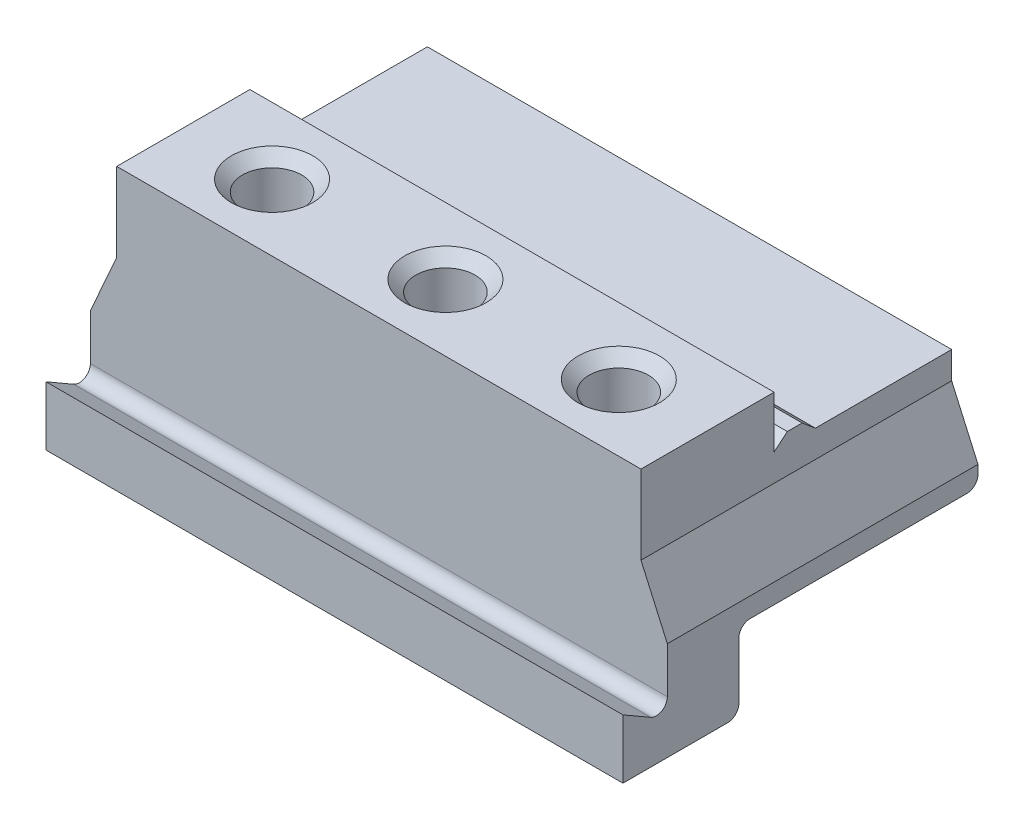
ISO-10303-21;
HEADER;
FILE_DESCRIPTION(('STEP AP214'),'2;1');
FILE_NAME('part.step','',(''),(''),'','','');
FILE_SCHEMA(('AUTOMOTIVE_DESIGN { 1 0 10303 214 1 1 1 1 }'));
ENDSEC;
DATA;
#1=APPLICATION_CONTEXT('core data for automotive mechanical design processes');
#2=APPLICATION_PROTOCOL_DEFINITION('international standard','automotive_design',2000,#1);
#3=PRODUCT_CONTEXT('',#1,'mechanical');
#4=PRODUCT('Part','Part','',(#3));
#5=PRODUCT_RELATED_PRODUCT_CATEGORY('part','',(#4));
#6=PRODUCT_DEFINITION_FORMATION('','',#4);
#7=PRODUCT_DEFINITION_CONTEXT('part definition',#1,'design');
#8=PRODUCT_DEFINITION('design','',#6,#7);
#9=PRODUCT_DEFINITION_SHAPE('','',#8);
#10=(LENGTH_UNIT() NAMED_UNIT(*) SI_UNIT(.MILLI.,.METRE.));
#11=(NAMED_UNIT(*) PLANE_ANGLE_UNIT() SI_UNIT($,.RADIAN.));
#12=(NAMED_UNIT(*) SI_UNIT($,.STERADIAN.) SOLID_ANGLE_UNIT());
#13=UNCERTAINTY_MEASURE_WITH_UNIT(LENGTH_MEASURE(1.E-05),#10,'distance_accuracy_value','');
#14=(GEOMETRIC_REPRESENTATION_CONTEXT(3) GLOBAL_UNCERTAINTY_ASSIGNED_CONTEXT((#13)) GLOBAL_UNIT_ASSIGNED_CONTEXT((#10,
#11,#12)) REPRESENTATION_CONTEXT('',''));
#15=CARTESIAN_POINT('',(0.,0.,0.));
#16=DIRECTION('',(0.,0.,1.));
#17=DIRECTION('',(1.,0.,0.));
#18=AXIS2_PLACEMENT_3D('',#15,#16,#17);
#19=CARTESIAN_POINT('',(78.,0.,-48.));
#20=DIRECTION('',(0.,-1.,0.));
#21=DIRECTION('',(1.,0.,0.));
#22=AXIS2_PLACEMENT_3D('',#19,#20,#21);
#23=PLANE('',#22);
#24=DIRECTION('',(0.,0.,1.));
#25=VECTOR('',#24,1.);
#26=CARTESIAN_POINT('',(0.,0.,-48.));
#27=LINE('',#26,#25);
#28=CARTESIAN_POINT('',(0.,0.,-14.1713819919104));
#29=VERTEX_POINT('',#28);
#30=CARTESIAN_POINT('',(0.,0.,0.));
#31=VERTEX_POINT('',#30);
#32=EDGE_CURVE('E197',#29,#31,#27,.T.);
#33=ORIENTED_EDGE('',*,*,#32,.F.);
#34=DIRECTION('',(1.,0.,0.));
#35=VECTOR('',#34,1.);
#36=CARTESIAN_POINT('',(-9.99999999999999,0.,-14.1713819919104));
#37=LINE('',#36,#35);
#38=CARTESIAN_POINT('',(78.,0.,-14.1713819919104));
#39=VERTEX_POINT('',#38);
#40=EDGE_CURVE('E409',#29,#39,#37,.T.);
#41=ORIENTED_EDGE('',*,*,#40,.T.);
#42=DIRECTION('',(0.,0.,1.));
#43=VECTOR('',#42,1.);
#44=CARTESIAN_POINT('',(78.,0.,-48.));
#45=LINE('',#44,#43);
#46=CARTESIAN_POINT('',(78.,0.,0.));
#47=VERTEX_POINT('',#46);
#48=EDGE_CURVE('E243',#39,#47,#45,.T.);
#49=ORIENTED_EDGE('',*,*,#48,.T.);
#50=DIRECTION('',(1.,0.,0.));
#51=VECTOR('',#50,1.);
#52=CARTESIAN_POINT('',(78.,0.,0.));
#53=LINE('',#52,#51);
#54=EDGE_CURVE('E213',#31,#47,#53,.T.);
#55=ORIENTED_EDGE('',*,*,#54,.F.);
#56=EDGE_LOOP('',(#33,#41,#49,#55));
#57=FACE_BOUND('',#56,.T.);
#58=ADVANCED_FACE('F41',(#57),#23,.T.);
#59=CARTESIAN_POINT('',(0.,0.,-48.));
#60=DIRECTION('',(-1.,0.,0.));
#61=DIRECTION('',(0.,0.,1.));
#62=AXIS2_PLACEMENT_3D('',#59,#60,#61);
#63=PLANE('',#62);
#64=DIRECTION('',(0.,-1.,0.));
#65=VECTOR('',#64,1.);
#66=CARTESIAN_POINT('',(0.,0.,-6.));
#67=LINE('',#66,#65);
#68=CARTESIAN_POINT('',(0.,13.33,-6.));
#69=VERTEX_POINT('',#68);
#70=CARTESIAN_POINT('',(0.,7.13397459621554,-6.));
#71=VERTEX_POINT('',#70);
#72=EDGE_CURVE('E490',#69,#71,#67,.T.);
#73=ORIENTED_EDGE('',*,*,#72,.F.);
#74=DIRECTION('',(0.,0.,1.));
#75=VECTOR('',#74,1.);
#76=CARTESIAN_POINT('',(0.,13.33,-48.));
#77=LINE('',#76,#75);
#78=CARTESIAN_POINT('',(0.,13.33,-48.));
#79=VERTEX_POINT('',#78);
#80=EDGE_CURVE('E224',#79,#69,#77,.T.);
#81=ORIENTED_EDGE('',*,*,#80,.F.);
#82=DIRECTION('',(0.,-1.,0.));
#83=VECTOR('',#82,1.);
#84=CARTESIAN_POINT('',(0.,0.,-48.));
#85=LINE('',#84,#83);
#86=CARTESIAN_POINT('',(0.,12.17,-48.));
#87=VERTEX_POINT('',#86);
#88=EDGE_CURVE('E242',#79,#87,#85,.T.);
#89=ORIENTED_EDGE('',*,*,#88,.T.);
#90=CARTESIAN_POINT('',(0.,12.17,-46.5));
#91=DIRECTION('',(-1.,0.,0.));
#92=DIRECTION('',(0.,0.,1.));
#93=AXIS2_PLACEMENT_3D('',#90,#91,#92);
#94=CIRCLE('',#93,1.5);
#95=CARTESIAN_POINT('',(0.,10.67,-46.5));
#96=VERTEX_POINT('',#95);
#97=EDGE_CURVE('E63',#96,#87,#94,.F.);
#98=ORIENTED_EDGE('',*,*,#97,.F.);
#99=DIRECTION('',(0.,0.,-1.));
#100=VECTOR('',#99,1.);
#101=CARTESIAN_POINT('',(0.,10.67,-48.));
#102=LINE('',#101,#100);
#103=CARTESIAN_POINT('',(0.,10.67,-17.1713819919104));
#104=VERTEX_POINT('',#103);
#105=EDGE_CURVE('E469',#104,#96,#102,.T.);
#106=ORIENTED_EDGE('',*,*,#105,.F.);
#107=CARTESIAN_POINT('',(0.,9.17,-17.1713819919104));
#108=DIRECTION('',(-1.,0.,0.));
#109=DIRECTION('',(0.,0.,1.));
#110=AXIS2_PLACEMENT_3D('',#107,#108,#109);
#111=CIRCLE('',#110,1.5);
#112=CARTESIAN_POINT('',(0.,9.16999999999999,-15.6713819919104));
#113=VERTEX_POINT('',#112);
#114=EDGE_CURVE('E472',#104,#113,#111,.F.);
#115=ORIENTED_EDGE('',*,*,#114,.T.);
#116=DIRECTION('',(0.,1.,0.));
#117=VECTOR('',#116,1.);
#118=CARTESIAN_POINT('',(0.,0.,-15.6713819919104));
#119=LINE('',#118,#117);
#120=CARTESIAN_POINT('',(0.,1.50000000000001,-15.6713819919104));
#121=VERTEX_POINT('',#120);
#122=EDGE_CURVE('E471',#121,#113,#119,.T.);
#123=ORIENTED_EDGE('',*,*,#122,.F.);
#124=CARTESIAN_POINT('',(0.,1.5,-14.1713819919104));
#125=DIRECTION('',(-1.,0.,0.));
#126=DIRECTION('',(0.,0.,1.));
#127=AXIS2_PLACEMENT_3D('',#124,#125,#126);
#128=CIRCLE('',#127,1.5);
#129=EDGE_CURVE('E479',#121,#29,#128,.T.);
#130=ORIENTED_EDGE('',*,*,#129,.T.);
#131=ORIENTED_EDGE('',*,*,#32,.T.);
#132=DIRECTION('',(0.,-1.,0.));
#133=VECTOR('',#132,1.);
#134=CARTESIAN_POINT('',(0.,0.,0.));
#135=LINE('',#134,#133);
#136=CARTESIAN_POINT('',(0.,8.,0.));
#137=VERTEX_POINT('',#136);
#138=EDGE_CURVE('E219',#137,#31,#135,.T.);
#139=ORIENTED_EDGE('',*,*,#138,.F.);
#140=DIRECTION('',(0.,0.500000000000004,0.866025403784436));
#141=VECTOR('',#140,1.);
#142=CARTESIAN_POINT('',(0.,-14.7846096908267,-39.4641016151376));
#143=LINE('',#142,#141);
#144=CARTESIAN_POINT('',(0.,5.83493649053889,-3.74999999999999));
#145=VERTEX_POINT('',#144);
#146=EDGE_CURVE('E191',#145,#137,#143,.T.);
#147=ORIENTED_EDGE('',*,*,#146,.F.);
#148=CARTESIAN_POINT('',(0.,7.13397459621554,-4.5));
#149=DIRECTION('',(-1.,0.,0.));
#150=DIRECTION('',(0.,0.,1.));
#151=AXIS2_PLACEMENT_3D('',#148,#149,#150);
#152=CIRCLE('',#151,1.5);
#153=EDGE_CURVE('E478',#71,#145,#152,.T.);
#154=ORIENTED_EDGE('',*,*,#153,.F.);
#155=EDGE_LOOP('',(#73,#81,#89,#98,#106,#115,#123,#130,#131,#139,#147,#154));
#156=FACE_BOUND('',#155,.T.);
#157=ADVANCED_FACE('F287',(#156),#63,.T.);
#158=CARTESIAN_POINT('',(78.,13.33,-48.));
#159=DIRECTION('',(1.,0.,0.));
#160=DIRECTION('',(0.,0.,-1.));
#161=AXIS2_PLACEMENT_3D('',#158,#159,#160);
#162=PLANE('',#161);
#163=DIRECTION('',(0.,1.,0.));
#164=VECTOR('',#163,1.);
#165=CARTESIAN_POINT('',(78.,7.13397459621554,-6.));
#166=LINE('',#165,#164);
#167=CARTESIAN_POINT('',(78.,7.13397459621554,-6.));
#168=VERTEX_POINT('',#167);
#169=CARTESIAN_POINT('',(78.,13.33,-6.));
#170=VERTEX_POINT('',#169);
#171=EDGE_CURVE('E423',#168,#170,#166,.T.);
#172=ORIENTED_EDGE('',*,*,#171,.F.);
#173=CARTESIAN_POINT('',(78.,7.13397459621554,-4.5));
#174=DIRECTION('',(1.,0.,0.));
#175=DIRECTION('',(0.,0.,-1.));
#176=AXIS2_PLACEMENT_3D('',#173,#174,#175);
#177=CIRCLE('',#176,1.5);
#178=CARTESIAN_POINT('',(78.,5.83493649053889,-3.74999999999999));
#179=VERTEX_POINT('',#178);
#180=EDGE_CURVE('E208',#179,#168,#177,.T.);
#181=ORIENTED_EDGE('',*,*,#180,.F.);
#182=DIRECTION('',(0.,-0.500000000000004,-0.866025403784436));
#183=VECTOR('',#182,1.);
#184=CARTESIAN_POINT('',(78.,8.,0.));
#185=LINE('',#184,#183);
#186=CARTESIAN_POINT('',(78.,8.,0.));
#187=VERTEX_POINT('',#186);
#188=EDGE_CURVE('E192',#187,#179,#185,.T.);
#189=ORIENTED_EDGE('',*,*,#188,.F.);
#190=DIRECTION('',(0.,1.,0.));
#191=VECTOR('',#190,1.);
#192=CARTESIAN_POINT('',(78.,13.33,0.));
#193=LINE('',#192,#191);
#194=EDGE_CURVE('E210',#47,#187,#193,.T.);
#195=ORIENTED_EDGE('',*,*,#194,.F.);
#196=ORIENTED_EDGE('',*,*,#48,.F.);
#197=CARTESIAN_POINT('',(78.,1.5,-14.1713819919104));
#198=DIRECTION('',(1.,0.,0.));
#199=DIRECTION('',(0.,0.,-1.));
#200=AXIS2_PLACEMENT_3D('',#197,#198,#199);
#201=CIRCLE('',#200,1.5);
#202=CARTESIAN_POINT('',(78.,1.50000000000001,-15.6713819919104));
#203=VERTEX_POINT('',#202);
#204=EDGE_CURVE('E444',#39,#203,#201,.T.);
#205=ORIENTED_EDGE('',*,*,#204,.T.);
#206=DIRECTION('',(0.,-1.,0.));
#207=VECTOR('',#206,1.);
#208=CARTESIAN_POINT('',(78.,9.16999999999999,-15.6713819919104));
#209=LINE('',#208,#207);
#210=CARTESIAN_POINT('',(78.,9.16999999999999,-15.6713819919104));
#211=VERTEX_POINT('',#210);
#212=EDGE_CURVE('E454',#211,#203,#209,.T.);
#213=ORIENTED_EDGE('',*,*,#212,.F.);
#214=CARTESIAN_POINT('',(78.,9.17,-17.1713819919104));
#215=DIRECTION('',(-1.,0.,0.));
#216=DIRECTION('',(0.,0.,1.));
#217=AXIS2_PLACEMENT_3D('',#214,#215,#216);
#218=CIRCLE('',#217,1.5);
#219=CARTESIAN_POINT('',(78.,10.67,-17.1713819919104));
#220=VERTEX_POINT('',#219);
#221=EDGE_CURVE('E459',#211,#220,#218,.T.);
#222=ORIENTED_EDGE('',*,*,#221,.T.);
#223=DIRECTION('',(0.,0.,1.));
#224=VECTOR('',#223,1.);
#225=CARTESIAN_POINT('',(78.,10.67,-46.5));
#226=LINE('',#225,#224);
#227=CARTESIAN_POINT('',(78.,10.67,-46.5));
#228=VERTEX_POINT('',#227);
#229=EDGE_CURVE('E458',#228,#220,#226,.T.);
#230=ORIENTED_EDGE('',*,*,#229,.F.);
#231=CARTESIAN_POINT('',(78.,12.17,-46.5));
#232=DIRECTION('',(-1.,0.,0.));
#233=DIRECTION('',(0.,0.,1.));
#234=AXIS2_PLACEMENT_3D('',#231,#232,#233);
#235=CIRCLE('',#234,1.5);
#236=CARTESIAN_POINT('',(78.,12.17,-48.));
#237=VERTEX_POINT('',#236);
#238=EDGE_CURVE('E445',#237,#228,#235,.T.);
#239=ORIENTED_EDGE('',*,*,#238,.F.);
#240=DIRECTION('',(0.,1.,0.));
#241=VECTOR('',#240,1.);
#242=CARTESIAN_POINT('',(78.,13.33,-48.));
#243=LINE('',#242,#241);
#244=CARTESIAN_POINT('',(78.,13.33,-48.));
#245=VERTEX_POINT('',#244);
#246=EDGE_CURVE('E220',#237,#245,#243,.T.);
#247=ORIENTED_EDGE('',*,*,#246,.T.);
#248=DIRECTION('',(0.,0.,1.));
#249=VECTOR('',#248,1.);
#250=CARTESIAN_POINT('',(78.,13.33,-48.));
#251=LINE('',#250,#249);
#252=EDGE_CURVE('E239',#245,#170,#251,.T.);
#253=ORIENTED_EDGE('',*,*,#252,.T.);
#254=EDGE_LOOP('',(#172,#181,#189,#195,#196,#205,#213,#222,#230,#239,#247,#253));
#255=FACE_BOUND('',#254,.T.);
#256=ADVANCED_FACE('F204',(#255),#162,.T.);
#257=CARTESIAN_POINT('',(0.,0.,-48.));
#258=DIRECTION('',(0.,0.,-1.));
#259=DIRECTION('',(-1.,0.,0.));
#260=AXIS2_PLACEMENT_3D('',#257,#258,#259);
#261=PLANE('',#260);
#262=DIRECTION('',(-1.,0.,0.));
#263=VECTOR('',#262,1.);
#264=CARTESIAN_POINT('',(0.,25.,-48.));
#265=LINE('',#264,#263);
#266=CARTESIAN_POINT('',(74.4381705175317,25.,-48.));
#267=VERTEX_POINT('',#266);
#268=CARTESIAN_POINT('',(3.5618294824683,25.,-48.));
#269=VERTEX_POINT('',#268);
#270=EDGE_CURVE('E250',#267,#269,#265,.T.);
#271=ORIENTED_EDGE('',*,*,#270,.F.);
#272=DIRECTION('',(0.,1.,0.));
#273=VECTOR('',#272,1.);
#274=CARTESIAN_POINT('',(74.4381705175317,32.,-48.));
#275=LINE('',#274,#273);
#276=CARTESIAN_POINT('',(74.4381705175317,21.33,-48.));
#277=VERTEX_POINT('',#276);
#278=EDGE_CURVE('E505',#277,#267,#275,.T.);
#279=ORIENTED_EDGE('',*,*,#278,.F.);
#280=DIRECTION('',(-0.4067366430758,0.913545457642601,0.));
#281=VECTOR('',#280,1.);
#282=CARTESIAN_POINT('',(74.4381705175317,21.33,-48.));
#283=LINE('',#282,#281);
#284=EDGE_CURVE('E497',#245,#277,#283,.T.);
#285=ORIENTED_EDGE('',*,*,#284,.F.);
#286=ORIENTED_EDGE('',*,*,#246,.F.);
#287=DIRECTION('',(1.,0.,0.));
#288=VECTOR('',#287,1.);
#289=CARTESIAN_POINT('',(-9.99999999999999,12.17,-48.));
#290=LINE('',#289,#288);
#291=EDGE_CURVE('E198',#237,#87,#290,.F.);
#292=ORIENTED_EDGE('',*,*,#291,.T.);
#293=ORIENTED_EDGE('',*,*,#88,.F.);
#294=DIRECTION('',(-0.406736643075801,-0.913545457642601,0.));
#295=VECTOR('',#294,1.);
#296=CARTESIAN_POINT('',(0.,13.33,-48.));
#297=LINE('',#296,#295);
#298=CARTESIAN_POINT('',(3.5618294824683,21.33,-48.));
#299=VERTEX_POINT('',#298);
#300=EDGE_CURVE('E510',#299,#79,#297,.T.);
#301=ORIENTED_EDGE('',*,*,#300,.F.);
#302=DIRECTION('',(0.,-1.,0.));
#303=VECTOR('',#302,1.);
#304=CARTESIAN_POINT('',(3.5618294824683,21.33,-48.));
#305=LINE('',#304,#303);
#306=EDGE_CURVE('E504',#269,#299,#305,.T.);
#307=ORIENTED_EDGE('',*,*,#306,.F.);
#308=EDGE_LOOP('',(#271,#279,#285,#286,#292,#293,#301,#307));
#309=FACE_BOUND('',#308,.T.);
#310=ADVANCED_FACE('F308',(#309),#261,.T.);
#311=CARTESIAN_POINT('',(0.,13.33,-48.));
#312=DIRECTION('',(-0.9135454576426,0.406736643075801,0.));
#313=DIRECTION('',(-0.406736643075801,-0.913545457642601,0.));
#314=AXIS2_PLACEMENT_3D('',#311,#312,#313);
#315=PLANE('',#314);
#316=DIRECTION('',(-0.406736643075801,-0.913545457642601,0.));
#317=VECTOR('',#316,1.);
#318=CARTESIAN_POINT('',(0.,13.33,-6.));
#319=LINE('',#318,#317);
#320=CARTESIAN_POINT('',(3.5618294824683,21.33,-6.));
#321=VERTEX_POINT('',#320);
#322=EDGE_CURVE('E487',#321,#69,#319,.T.);
#323=ORIENTED_EDGE('',*,*,#322,.F.);
#324=DIRECTION('',(0.,0.,1.));
#325=VECTOR('',#324,1.);
#326=CARTESIAN_POINT('',(3.5618294824683,21.33,-48.));
#327=LINE('',#326,#325);
#328=EDGE_CURVE('E226',#299,#321,#327,.T.);
#329=ORIENTED_EDGE('',*,*,#328,.F.);
#330=ORIENTED_EDGE('',*,*,#300,.T.);
#331=ORIENTED_EDGE('',*,*,#80,.T.);
#332=EDGE_LOOP('',(#323,#329,#330,#331));
#333=FACE_BOUND('',#332,.T.);
#334=ADVANCED_FACE('F321',(#333),#315,.T.);
#335=CARTESIAN_POINT('',(3.5618294824683,21.33,-48.));
#336=DIRECTION('',(-1.,0.,0.));
#337=DIRECTION('',(0.,0.,1.));
#338=AXIS2_PLACEMENT_3D('',#335,#336,#337);
#339=PLANE('',#338);
#340=DIRECTION('',(0.,-1.,0.));
#341=VECTOR('',#340,1.);
#342=CARTESIAN_POINT('',(3.5618294824683,21.33,-6.));
#343=LINE('',#342,#341);
#344=CARTESIAN_POINT('',(3.5618294824683,32.,-6.));
#345=VERTEX_POINT('',#344);
#346=EDGE_CURVE('E484',#345,#321,#343,.T.);
#347=ORIENTED_EDGE('',*,*,#346,.F.);
#348=DIRECTION('',(0.,0.,1.));
#349=VECTOR('',#348,1.);
#350=CARTESIAN_POINT('',(3.5618294824683,32.,-48.));
#351=LINE('',#350,#349);
#352=CARTESIAN_POINT('',(3.5618294824683,32.,-24.));
#353=VERTEX_POINT('',#352);
#354=EDGE_CURVE('E233',#353,#345,#351,.T.);
#355=ORIENTED_EDGE('',*,*,#354,.F.);
#356=DIRECTION('',(0.,1.,0.));
#357=VECTOR('',#356,1.);
#358=CARTESIAN_POINT('',(3.5618294824683,21.33,-24.));
#359=LINE('',#358,#357);
#360=CARTESIAN_POINT('',(3.5618294824683,25.,-24.));
#361=VERTEX_POINT('',#360);
#362=EDGE_CURVE('E493',#361,#353,#359,.T.);
#363=ORIENTED_EDGE('',*,*,#362,.F.);
#364=DIRECTION('',(0.,-0.642787609686541,0.766044443118977));
#365=VECTOR('',#364,1.);
#366=CARTESIAN_POINT('',(3.5618294824683,35.3013374421653,-36.2766559052257));
#367=LINE('',#366,#365);
#368=CARTESIAN_POINT('',(3.5618294824683,26.5,-25.7876303888913));
#369=VERTEX_POINT('',#368);
#370=EDGE_CURVE('E491',#369,#361,#367,.T.);
#371=ORIENTED_EDGE('',*,*,#370,.F.);
#372=DIRECTION('',(0.,0.,1.));
#373=VECTOR('',#372,1.);
#374=CARTESIAN_POINT('',(3.5618294824683,26.5,-48.));
#375=LINE('',#374,#373);
#376=CARTESIAN_POINT('',(3.5618294824683,26.5,-27.7876303888913));
#377=VERTEX_POINT('',#376);
#378=EDGE_CURVE('E492',#377,#369,#375,.T.);
#379=ORIENTED_EDGE('',*,*,#378,.F.);
#380=DIRECTION('',(0.,0.642787609686539,0.766044443118978));
#381=VECTOR('',#380,1.);
#382=CARTESIAN_POINT('',(3.5618294824683,14.4112313893849,-42.1944638106319));
#383=LINE('',#382,#381);
#384=CARTESIAN_POINT('',(3.5618294824683,25.,-29.5752607777826));
#385=VERTEX_POINT('',#384);
#386=EDGE_CURVE('E217',#385,#377,#383,.T.);
#387=ORIENTED_EDGE('',*,*,#386,.F.);
#388=DIRECTION('',(0.,0.,1.));
#389=VECTOR('',#388,1.);
#390=CARTESIAN_POINT('',(3.5618294824683,25.,-48.));
#391=LINE('',#390,#389);
#392=EDGE_CURVE('E470',#269,#385,#391,.T.);
#393=ORIENTED_EDGE('',*,*,#392,.F.);
#394=ORIENTED_EDGE('',*,*,#306,.T.);
#395=ORIENTED_EDGE('',*,*,#328,.T.);
#396=EDGE_LOOP('',(#347,#355,#363,#371,#379,#387,#393,#394,#395));
#397=FACE_BOUND('',#396,.T.);
#398=ADVANCED_FACE('F318',(#397),#339,.T.);
#399=CARTESIAN_POINT('',(3.5618294824683,32.,-48.));
#400=DIRECTION('',(0.,1.,0.));
#401=DIRECTION('',(0.,0.,1.));
#402=AXIS2_PLACEMENT_3D('',#399,#400,#401);
#403=PLANE('',#402);
#404=CARTESIAN_POINT('',(62.4381705175317,32.,-15.));
#405=DIRECTION('',(0.,1.,0.));
#406=DIRECTION('',(0.,0.,1.));
#407=AXIS2_PLACEMENT_3D('',#404,#405,#406);
#408=CIRCLE('',#407,5.5);
#409=CARTESIAN_POINT('',(62.4381705175317,32.,-9.49999999999999));
#410=VERTEX_POINT('',#409);
#411=EDGE_CURVE('E266',#410,#410,#408,.F.);
#412=ORIENTED_EDGE('',*,*,#411,.T.);
#413=EDGE_LOOP('',(#412));
#414=FACE_BOUND('',#413,.T.);
#415=CARTESIAN_POINT('',(39.,32.,-15.));
#416=DIRECTION('',(0.,1.,0.));
#417=DIRECTION('',(0.,0.,1.));
#418=AXIS2_PLACEMENT_3D('',#415,#416,#417);
#419=CIRCLE('',#418,5.49999999999998);
#420=CARTESIAN_POINT('',(39.,32.,-9.50000000000002));
#421=VERTEX_POINT('',#420);
#422=EDGE_CURVE('E265',#421,#421,#419,.F.);
#423=ORIENTED_EDGE('',*,*,#422,.T.);
#424=EDGE_LOOP('',(#423));
#425=FACE_BOUND('',#424,.T.);
#426=CARTESIAN_POINT('',(15.5618294824683,32.,-15.));
#427=DIRECTION('',(0.,1.,0.));
#428=DIRECTION('',(0.,0.,1.));
#429=AXIS2_PLACEMENT_3D('',#426,#427,#428);
#430=CIRCLE('',#429,5.49999999999998);
#431=CARTESIAN_POINT('',(15.5618294824683,32.,-9.50000000000002));
#432=VERTEX_POINT('',#431);
#433=EDGE_CURVE('E258',#432,#432,#430,.F.);
#434=ORIENTED_EDGE('',*,*,#433,.T.);
#435=EDGE_LOOP('',(#434));
#436=FACE_BOUND('',#435,.T.);
#437=DIRECTION('',(1.,0.,0.));
#438=VECTOR('',#437,1.);
#439=CARTESIAN_POINT('',(-9.99999999999999,32.,-6.));
#440=LINE('',#439,#438);
#441=CARTESIAN_POINT('',(74.4381705175317,32.,-6.));
#442=VERTEX_POINT('',#441);
#443=EDGE_CURVE('E425',#345,#442,#440,.T.);
#444=ORIENTED_EDGE('',*,*,#443,.T.);
#445=DIRECTION('',(0.,0.,1.));
#446=VECTOR('',#445,1.);
#447=CARTESIAN_POINT('',(74.4381705175317,32.,-48.));
#448=LINE('',#447,#446);
#449=CARTESIAN_POINT('',(74.4381705175317,32.,-24.));
#450=VERTEX_POINT('',#449);
#451=EDGE_CURVE('E234',#450,#442,#448,.T.);
#452=ORIENTED_EDGE('',*,*,#451,.F.);
#453=DIRECTION('',(1.,0.,0.));
#454=VECTOR('',#453,1.);
#455=CARTESIAN_POINT('',(-9.99999999999999,32.,-24.));
#456=LINE('',#455,#454);
#457=EDGE_CURVE('E212',#353,#450,#456,.T.);
#458=ORIENTED_EDGE('',*,*,#457,.F.);
#459=ORIENTED_EDGE('',*,*,#354,.T.);
#460=EDGE_LOOP('',(#444,#452,#458,#459));
#461=FACE_BOUND('',#460,.T.);
#462=ADVANCED_FACE('F317',(#414,#425,#436,#461),#403,.T.);
#463=CARTESIAN_POINT('',(74.4381705175317,32.,-48.));
#464=DIRECTION('',(1.,0.,0.));
#465=DIRECTION('',(0.,0.,-1.));
#466=AXIS2_PLACEMENT_3D('',#463,#464,#465);
#467=PLANE('',#466);
#468=DIRECTION('',(0.,1.,0.));
#469=VECTOR('',#468,1.);
#470=CARTESIAN_POINT('',(74.4381705175317,32.,-6.));
#471=LINE('',#470,#469);
#472=CARTESIAN_POINT('',(74.4381705175317,21.33,-6.));
#473=VERTEX_POINT('',#472);
#474=EDGE_CURVE('E483',#473,#442,#471,.T.);
#475=ORIENTED_EDGE('',*,*,#474,.F.);
#476=DIRECTION('',(0.,0.,1.));
#477=VECTOR('',#476,1.);
#478=CARTESIAN_POINT('',(74.4381705175317,21.33,-48.));
#479=LINE('',#478,#477);
#480=EDGE_CURVE('E240',#277,#473,#479,.T.);
#481=ORIENTED_EDGE('',*,*,#480,.F.);
#482=ORIENTED_EDGE('',*,*,#278,.T.);
#483=DIRECTION('',(0.,0.,-1.));
#484=VECTOR('',#483,1.);
#485=CARTESIAN_POINT('',(74.4381705175317,25.,-48.));
#486=LINE('',#485,#484);
#487=CARTESIAN_POINT('',(74.4381705175317,25.,-29.5752607777826));
#488=VERTEX_POINT('',#487);
#489=EDGE_CURVE('E60',#488,#267,#486,.T.);
#490=ORIENTED_EDGE('',*,*,#489,.F.);
#491=DIRECTION('',(0.,-0.642787609686539,-0.766044443118978));
#492=VECTOR('',#491,1.);
#493=CARTESIAN_POINT('',(74.4381705175317,18.8198183615318,-36.9405144483118));
#494=LINE('',#493,#492);
#495=CARTESIAN_POINT('',(74.4381705175317,26.5,-27.7876303888913));
#496=VERTEX_POINT('',#495);
#497=EDGE_CURVE('E253',#496,#488,#494,.T.);
#498=ORIENTED_EDGE('',*,*,#497,.F.);
#499=DIRECTION('',(0.,0.,-1.));
#500=VECTOR('',#499,1.);
#501=CARTESIAN_POINT('',(74.4381705175317,26.5,-48.));
#502=LINE('',#501,#500);
#503=CARTESIAN_POINT('',(74.4381705175317,26.5,-25.7876303888913));
#504=VERTEX_POINT('',#503);
#505=EDGE_CURVE('E254',#504,#496,#502,.T.);
#506=ORIENTED_EDGE('',*,*,#505,.F.);
#507=DIRECTION('',(0.,0.642787609686541,-0.766044443118977));
#508=VECTOR('',#507,1.);
#509=CARTESIAN_POINT('',(74.4381705175317,39.7099244143123,-41.5306052675459));
#510=LINE('',#509,#508);
#511=CARTESIAN_POINT('',(74.4381705175317,25.,-24.));
#512=VERTEX_POINT('',#511);
#513=EDGE_CURVE('E252',#512,#504,#510,.T.);
#514=ORIENTED_EDGE('',*,*,#513,.F.);
#515=DIRECTION('',(0.,-1.,0.));
#516=VECTOR('',#515,1.);
#517=CARTESIAN_POINT('',(74.4381705175317,32.,-24.));
#518=LINE('',#517,#516);
#519=EDGE_CURVE('E248',#450,#512,#518,.T.);
#520=ORIENTED_EDGE('',*,*,#519,.F.);
#521=ORIENTED_EDGE('',*,*,#451,.T.);
#522=EDGE_LOOP('',(#475,#481,#482,#490,#498,#506,#514,#520,#521));
#523=FACE_BOUND('',#522,.T.);
#524=ADVANCED_FACE('F315',(#523),#467,.T.);
#525=CARTESIAN_POINT('',(74.4381705175317,21.33,-48.));
#526=DIRECTION('',(0.913545457642601,0.4067366430758,0.));
#527=DIRECTION('',(-0.4067366430758,0.913545457642601,0.));
#528=AXIS2_PLACEMENT_3D('',#525,#526,#527);
#529=PLANE('',#528);
#530=DIRECTION('',(-0.4067366430758,0.913545457642601,0.));
#531=VECTOR('',#530,1.);
#532=CARTESIAN_POINT('',(74.4381705175317,21.33,-6.));
#533=LINE('',#532,#531);
#534=EDGE_CURVE('E481',#170,#473,#533,.T.);
#535=ORIENTED_EDGE('',*,*,#534,.F.);
#536=ORIENTED_EDGE('',*,*,#252,.F.);
#537=ORIENTED_EDGE('',*,*,#284,.T.);
#538=ORIENTED_EDGE('',*,*,#480,.T.);
#539=EDGE_LOOP('',(#535,#536,#537,#538));
#540=FACE_BOUND('',#539,.T.);
#541=ADVANCED_FACE('F307',(#540),#529,.T.);
#542=CARTESIAN_POINT('',(0.,0.,0.));
#543=DIRECTION('',(0.,0.,-1.));
#544=DIRECTION('',(-1.,0.,0.));
#545=AXIS2_PLACEMENT_3D('',#542,#543,#544);
#546=PLANE('',#545);
#547=ORIENTED_EDGE('',*,*,#194,.T.);
#548=DIRECTION('',(-1.,0.,0.));
#549=VECTOR('',#548,1.);
#550=CARTESIAN_POINT('',(0.,8.,0.));
#551=LINE('',#550,#549);
#552=EDGE_CURVE('E190',#187,#137,#551,.T.);
#553=ORIENTED_EDGE('',*,*,#552,.T.);
#554=ORIENTED_EDGE('',*,*,#138,.T.);
#555=ORIENTED_EDGE('',*,*,#54,.T.);
#556=EDGE_LOOP('',(#547,#553,#554,#555));
#557=FACE_BOUND('',#556,.T.);
#558=ADVANCED_FACE('F214',(#557),#546,.F.);
#559=CARTESIAN_POINT('',(-9.99999999999999,7.13397459621554,-6.));
#560=DIRECTION('',(0.,0.,-1.));
#561=DIRECTION('',(-1.,0.,0.));
#562=AXIS2_PLACEMENT_3D('',#559,#560,#561);
#563=PLANE('',#562);
#564=ORIENTED_EDGE('',*,*,#72,.T.);
#565=DIRECTION('',(1.,0.,0.));
#566=VECTOR('',#565,1.);
#567=CARTESIAN_POINT('',(-9.99999999999999,7.13397459621554,-6.));
#568=LINE('',#567,#566);
#569=EDGE_CURVE('E430',#71,#168,#568,.T.);
#570=ORIENTED_EDGE('',*,*,#569,.T.);
#571=ORIENTED_EDGE('',*,*,#171,.T.);
#572=ORIENTED_EDGE('',*,*,#534,.T.);
#573=ORIENTED_EDGE('',*,*,#474,.T.);
#574=ORIENTED_EDGE('',*,*,#443,.F.);
#575=ORIENTED_EDGE('',*,*,#346,.T.);
#576=ORIENTED_EDGE('',*,*,#322,.T.);
#577=EDGE_LOOP('',(#564,#570,#571,#572,#573,#574,#575,#576));
#578=FACE_BOUND('',#577,.T.);
#579=ADVANCED_FACE('F331',(#578),#563,.F.);
#580=CARTESIAN_POINT('',(-9.99999999999999,7.13397459621554,-4.5));
#581=DIRECTION('',(1.,0.,0.));
#582=DIRECTION('',(0.,0.,-1.));
#583=AXIS2_PLACEMENT_3D('',#580,#581,#582);
#584=CYLINDRICAL_SURFACE('',#583,1.5);
#585=ORIENTED_EDGE('',*,*,#153,.T.);
#586=DIRECTION('',(1.,0.,0.));
#587=VECTOR('',#586,1.);
#588=CARTESIAN_POINT('',(-9.99999999999999,5.83493649053889,-3.74999999999999));
#589=LINE('',#588,#587);
#590=EDGE_CURVE('E421',#145,#179,#589,.T.);
#591=ORIENTED_EDGE('',*,*,#590,.T.);
#592=ORIENTED_EDGE('',*,*,#180,.T.);
#593=ORIENTED_EDGE('',*,*,#569,.F.);
#594=EDGE_LOOP('',(#585,#591,#592,#593));
#595=FACE_BOUND('',#594,.T.);
#596=ADVANCED_FACE('F376',(#595),#584,.F.);
#597=CARTESIAN_POINT('',(-9.99999999999999,8.,0.));
#598=DIRECTION('',(0.,-0.866025403784436,0.500000000000004));
#599=DIRECTION('',(0.,-0.500000000000004,-0.866025403784436));
#600=AXIS2_PLACEMENT_3D('',#597,#598,#599);
#601=PLANE('',#600);
#602=ORIENTED_EDGE('',*,*,#146,.T.);
#603=ORIENTED_EDGE('',*,*,#552,.F.);
#604=ORIENTED_EDGE('',*,*,#188,.T.);
#605=ORIENTED_EDGE('',*,*,#590,.F.);
#606=EDGE_LOOP('',(#602,#603,#604,#605));
#607=FACE_BOUND('',#606,.T.);
#608=ADVANCED_FACE('F186',(#607),#601,.F.);
#609=CARTESIAN_POINT('',(-9.99999999999999,1.5,-14.1713819919104));
#610=DIRECTION('',(1.,0.,0.));
#611=DIRECTION('',(0.,0.,-1.));
#612=AXIS2_PLACEMENT_3D('',#609,#610,#611);
#613=CYLINDRICAL_SURFACE('',#612,1.5);
#614=DIRECTION('',(1.,0.,0.));
#615=VECTOR('',#614,1.);
#616=CARTESIAN_POINT('',(-9.99999999999999,1.50000000000001,-15.6713819919104));
#617=LINE('',#616,#615);
#618=EDGE_CURVE('E411',#121,#203,#617,.T.);
#619=ORIENTED_EDGE('',*,*,#618,.T.);
#620=ORIENTED_EDGE('',*,*,#204,.F.);
#621=ORIENTED_EDGE('',*,*,#40,.F.);
#622=ORIENTED_EDGE('',*,*,#129,.F.);
#623=EDGE_LOOP('',(#619,#620,#621,#622));
#624=FACE_BOUND('',#623,.T.);
#625=ADVANCED_FACE('F334',(#624),#613,.T.);
#626=CARTESIAN_POINT('',(-9.99999999999999,9.16999999999999,-15.6713819919104));
#627=DIRECTION('',(0.,0.,1.));
#628=DIRECTION('',(1.,0.,0.));
#629=AXIS2_PLACEMENT_3D('',#626,#627,#628);
#630=PLANE('',#629);
#631=ORIENTED_EDGE('',*,*,#122,.T.);
#632=DIRECTION('',(1.,0.,0.));
#633=VECTOR('',#632,1.);
#634=CARTESIAN_POINT('',(-9.99999999999999,9.16999999999999,-15.6713819919104));
#635=LINE('',#634,#633);
#636=EDGE_CURVE('E449',#113,#211,#635,.T.);
#637=ORIENTED_EDGE('',*,*,#636,.T.);
#638=ORIENTED_EDGE('',*,*,#212,.T.);
#639=ORIENTED_EDGE('',*,*,#618,.F.);
#640=EDGE_LOOP('',(#631,#637,#638,#639));
#641=FACE_BOUND('',#640,.T.);
#642=ADVANCED_FACE('F336',(#641),#630,.F.);
#643=CARTESIAN_POINT('',(-9.99999999999999,9.17,-17.1713819919104));
#644=DIRECTION('',(1.,0.,0.));
#645=DIRECTION('',(0.,0.,-1.));
#646=AXIS2_PLACEMENT_3D('',#643,#644,#645);
#647=CYLINDRICAL_SURFACE('',#646,1.5);
#648=DIRECTION('',(1.,0.,0.));
#649=VECTOR('',#648,1.);
#650=CARTESIAN_POINT('',(-9.99999999999999,10.67,-17.1713819919104));
#651=LINE('',#650,#649);
#652=EDGE_CURVE('E447',#104,#220,#651,.T.);
#653=ORIENTED_EDGE('',*,*,#652,.T.);
#654=ORIENTED_EDGE('',*,*,#221,.F.);
#655=ORIENTED_EDGE('',*,*,#636,.F.);
#656=ORIENTED_EDGE('',*,*,#114,.F.);
#657=EDGE_LOOP('',(#653,#654,#655,#656));
#658=FACE_BOUND('',#657,.T.);
#659=ADVANCED_FACE('F345',(#658),#647,.F.);
#660=CARTESIAN_POINT('',(-9.99999999999999,10.67,-46.5));
#661=DIRECTION('',(0.,1.,0.));
#662=DIRECTION('',(0.,0.,1.));
#663=AXIS2_PLACEMENT_3D('',#660,#661,#662);
#664=PLANE('',#663);
#665=ORIENTED_EDGE('',*,*,#105,.T.);
#666=DIRECTION('',(1.,0.,0.));
#667=VECTOR('',#666,1.);
#668=CARTESIAN_POINT('',(-9.99999999999999,10.67,-46.5));
#669=LINE('',#668,#667);
#670=EDGE_CURVE('E442',#96,#228,#669,.T.);
#671=ORIENTED_EDGE('',*,*,#670,.T.);
#672=ORIENTED_EDGE('',*,*,#229,.T.);
#673=ORIENTED_EDGE('',*,*,#652,.F.);
#674=EDGE_LOOP('',(#665,#671,#672,#673));
#675=FACE_BOUND('',#674,.T.);
#676=ADVANCED_FACE('F349',(#675),#664,.F.);
#677=CARTESIAN_POINT('',(-9.99999999999999,12.17,-46.5));
#678=DIRECTION('',(1.,0.,0.));
#679=DIRECTION('',(0.,0.,-1.));
#680=AXIS2_PLACEMENT_3D('',#677,#678,#679);
#681=CYLINDRICAL_SURFACE('',#680,1.5);
#682=ORIENTED_EDGE('',*,*,#97,.T.);
#683=ORIENTED_EDGE('',*,*,#291,.F.);
#684=ORIENTED_EDGE('',*,*,#238,.T.);
#685=ORIENTED_EDGE('',*,*,#670,.F.);
#686=EDGE_LOOP('',(#682,#683,#684,#685));
#687=FACE_BOUND('',#686,.T.);
#688=ADVANCED_FACE('F347',(#687),#681,.T.);
#689=CARTESIAN_POINT('',(-9.99999999999999,25.,-29.5752607777826));
#690=DIRECTION('',(0.,-1.,0.));
#691=DIRECTION('',(0.,0.,-1.));
#692=AXIS2_PLACEMENT_3D('',#689,#690,#691);
#693=PLANE('',#692);
#694=ORIENTED_EDGE('',*,*,#392,.T.);
#695=DIRECTION('',(1.,0.,0.));
#696=VECTOR('',#695,1.);
#697=CARTESIAN_POINT('',(-9.99999999999999,25.,-29.5752607777826));
#698=LINE('',#697,#696);
#699=EDGE_CURVE('E439',#385,#488,#698,.T.);
#700=ORIENTED_EDGE('',*,*,#699,.T.);
#701=ORIENTED_EDGE('',*,*,#489,.T.);
#702=ORIENTED_EDGE('',*,*,#270,.T.);
#703=EDGE_LOOP('',(#694,#700,#701,#702));
#704=FACE_BOUND('',#703,.T.);
#705=ADVANCED_FACE('F352',(#704),#693,.F.);
#706=CARTESIAN_POINT('',(-9.99999999999999,26.5,-27.7876303888913));
#707=DIRECTION('',(0.,-0.766044443118978,0.642787609686539));
#708=DIRECTION('',(0.,-0.642787609686539,-0.766044443118978));
#709=AXIS2_PLACEMENT_3D('',#706,#707,#708);
#710=PLANE('',#709);
#711=ORIENTED_EDGE('',*,*,#386,.T.);
#712=DIRECTION('',(1.,0.,0.));
#713=VECTOR('',#712,1.);
#714=CARTESIAN_POINT('',(-9.99999999999999,26.5,-27.7876303888913));
#715=LINE('',#714,#713);
#716=EDGE_CURVE('E440',#377,#496,#715,.T.);
#717=ORIENTED_EDGE('',*,*,#716,.T.);
#718=ORIENTED_EDGE('',*,*,#497,.T.);
#719=ORIENTED_EDGE('',*,*,#699,.F.);
#720=EDGE_LOOP('',(#711,#717,#718,#719));
#721=FACE_BOUND('',#720,.T.);
#722=ADVANCED_FACE('F357',(#721),#710,.F.);
#723=CARTESIAN_POINT('',(-9.99999999999999,26.5,-25.7876303888913));
#724=DIRECTION('',(0.,-1.,0.));
#725=DIRECTION('',(0.,0.,-1.));
#726=AXIS2_PLACEMENT_3D('',#723,#724,#725);
#727=PLANE('',#726);
#728=ORIENTED_EDGE('',*,*,#378,.T.);
#729=DIRECTION('',(1.,0.,0.));
#730=VECTOR('',#729,1.);
#731=CARTESIAN_POINT('',(-9.99999999999999,26.5,-25.7876303888913));
#732=LINE('',#731,#730);
#733=EDGE_CURVE('E432',#369,#504,#732,.T.);
#734=ORIENTED_EDGE('',*,*,#733,.T.);
#735=ORIENTED_EDGE('',*,*,#505,.T.);
#736=ORIENTED_EDGE('',*,*,#716,.F.);
#737=EDGE_LOOP('',(#728,#734,#735,#736));
#738=FACE_BOUND('',#737,.T.);
#739=ADVANCED_FACE('F359',(#738),#727,.F.);
#740=CARTESIAN_POINT('',(-9.99999999999999,25.,-24.));
#741=DIRECTION('',(0.,-0.766044443118977,-0.642787609686541));
#742=DIRECTION('',(0.,0.642787609686541,-0.766044443118977));
#743=AXIS2_PLACEMENT_3D('',#740,#741,#742);
#744=PLANE('',#743);
#745=ORIENTED_EDGE('',*,*,#370,.T.);
#746=DIRECTION('',(1.,0.,0.));
#747=VECTOR('',#746,1.);
#748=CARTESIAN_POINT('',(-9.99999999999999,25.,-24.));
#749=LINE('',#748,#747);
#750=EDGE_CURVE('E431',#361,#512,#749,.T.);
#751=ORIENTED_EDGE('',*,*,#750,.T.);
#752=ORIENTED_EDGE('',*,*,#513,.T.);
#753=ORIENTED_EDGE('',*,*,#733,.F.);
#754=EDGE_LOOP('',(#745,#751,#752,#753));
#755=FACE_BOUND('',#754,.T.);
#756=ADVANCED_FACE('F364',(#755),#744,.F.);
#757=CARTESIAN_POINT('',(-9.99999999999999,32.,-24.));
#758=DIRECTION('',(0.,0.,1.));
#759=DIRECTION('',(1.,0.,0.));
#760=AXIS2_PLACEMENT_3D('',#757,#758,#759);
#761=PLANE('',#760);
#762=ORIENTED_EDGE('',*,*,#362,.T.);
#763=ORIENTED_EDGE('',*,*,#457,.T.);
#764=ORIENTED_EDGE('',*,*,#519,.T.);
#765=ORIENTED_EDGE('',*,*,#750,.F.);
#766=EDGE_LOOP('',(#762,#763,#764,#765));
#767=FACE_BOUND('',#766,.T.);
#768=ADVANCED_FACE('F368',(#767),#761,.F.);
#769=CARTESIAN_POINT('',(15.5618294824683,22.,-15.));
#770=DIRECTION('',(0.,1.,0.));
#771=DIRECTION('',(0.,0.,1.));
#772=AXIS2_PLACEMENT_3D('',#769,#770,#771);
#773=CYLINDRICAL_SURFACE('',#772,4.);
#774=CARTESIAN_POINT('',(15.5618294824683,30.5,-15.));
#775=DIRECTION('',(0.,1.,0.));
#776=DIRECTION('',(0.,0.,1.));
#777=AXIS2_PLACEMENT_3D('',#774,#775,#776);
#778=CIRCLE('',#777,4.);
#779=CARTESIAN_POINT('',(15.5618294824683,30.5,-11.));
#780=VERTEX_POINT('',#779);
#781=EDGE_CURVE('E11',#780,#780,#778,.T.);
#782=ORIENTED_EDGE('',*,*,#781,.T.);
#783=EDGE_LOOP('',(#782));
#784=FACE_BOUND('',#783,.T.);
#785=CARTESIAN_POINT('',(15.5618294824683,22.,-15.));
#786=DIRECTION('',(0.,1.,0.));
#787=DIRECTION('',(0.,0.,1.));
#788=AXIS2_PLACEMENT_3D('',#785,#786,#787);
#789=CIRCLE('',#788,4.);
#790=CARTESIAN_POINT('',(15.5618294824683,22.,-11.));
#791=VERTEX_POINT('',#790);
#792=EDGE_CURVE('E412',#791,#791,#789,.T.);
#793=ORIENTED_EDGE('',*,*,#792,.F.);
#794=EDGE_LOOP('',(#793));
#795=FACE_BOUND('',#794,.T.);
#796=ADVANCED_FACE('F375',(#784,#795),#773,.F.);
#797=CARTESIAN_POINT('',(15.5618294824683,22.,-15.));
#798=DIRECTION('',(0.,1.,0.));
#799=DIRECTION('',(0.,0.,1.));
#800=AXIS2_PLACEMENT_3D('',#797,#798,#799);
#801=PLANE('',#800);
#802=ORIENTED_EDGE('',*,*,#792,.T.);
#803=EDGE_LOOP('',(#802));
#804=FACE_BOUND('',#803,.T.);
#805=ADVANCED_FACE('F384',(#804),#801,.T.);
#806=CARTESIAN_POINT('',(39.,22.,-15.));
#807=DIRECTION('',(0.,1.,0.));
#808=DIRECTION('',(0.,0.,1.));
#809=AXIS2_PLACEMENT_3D('',#806,#807,#808);
#810=CYLINDRICAL_SURFACE('',#809,4.);
#811=CARTESIAN_POINT('',(39.,30.5,-15.));
#812=DIRECTION('',(0.,1.,0.));
#813=DIRECTION('',(0.,0.,1.));
#814=AXIS2_PLACEMENT_3D('',#811,#812,#813);
#815=CIRCLE('',#814,4.);
#816=CARTESIAN_POINT('',(39.,30.5,-11.));
#817=VERTEX_POINT('',#816);
#818=EDGE_CURVE('E49',#817,#817,#815,.T.);
#819=ORIENTED_EDGE('',*,*,#818,.T.);
#820=EDGE_LOOP('',(#819));
#821=FACE_BOUND('',#820,.T.);
#822=CARTESIAN_POINT('',(39.,22.,-15.));
#823=DIRECTION('',(0.,1.,0.));
#824=DIRECTION('',(0.,0.,1.));
#825=AXIS2_PLACEMENT_3D('',#822,#823,#824);
#826=CIRCLE('',#825,4.);
#827=CARTESIAN_POINT('',(39.,22.,-11.));
#828=VERTEX_POINT('',#827);
#829=EDGE_CURVE('E406',#828,#828,#826,.T.);
#830=ORIENTED_EDGE('',*,*,#829,.F.);
#831=EDGE_LOOP('',(#830));
#832=FACE_BOUND('',#831,.T.);
#833=ADVANCED_FACE('F272',(#821,#832),#810,.F.);
#834=CARTESIAN_POINT('',(39.,22.,-15.));
#835=DIRECTION('',(0.,1.,0.));
#836=DIRECTION('',(0.,0.,1.));
#837=AXIS2_PLACEMENT_3D('',#834,#835,#836);
#838=PLANE('',#837);
#839=ORIENTED_EDGE('',*,*,#829,.T.);
#840=EDGE_LOOP('',(#839));
#841=FACE_BOUND('',#840,.T.);
#842=ADVANCED_FACE('F388',(#841),#838,.T.);
#843=CARTESIAN_POINT('',(62.4381705175317,22.,-15.));
#844=DIRECTION('',(0.,1.,0.));
#845=DIRECTION('',(0.,0.,1.));
#846=AXIS2_PLACEMENT_3D('',#843,#844,#845);
#847=CYLINDRICAL_SURFACE('',#846,4.00000000000001);
#848=CARTESIAN_POINT('',(62.4381705175317,30.5,-15.));
#849=DIRECTION('',(0.,1.,0.));
#850=DIRECTION('',(0.,0.,1.));
#851=AXIS2_PLACEMENT_3D('',#848,#849,#850);
#852=CIRCLE('',#851,4.00000000000001);
#853=CARTESIAN_POINT('',(62.4381705175317,30.5,-11.));
#854=VERTEX_POINT('',#853);
#855=EDGE_CURVE('E260',#854,#854,#852,.T.);
#856=ORIENTED_EDGE('',*,*,#855,.T.);
#857=EDGE_LOOP('',(#856));
#858=FACE_BOUND('',#857,.T.);
#859=CARTESIAN_POINT('',(62.4381705175317,22.,-15.));
#860=DIRECTION('',(0.,1.,0.));
#861=DIRECTION('',(0.,0.,1.));
#862=AXIS2_PLACEMENT_3D('',#859,#860,#861);
#863=CIRCLE('',#862,4.00000000000001);
#864=CARTESIAN_POINT('',(62.4381705175317,22.,-11.));
#865=VERTEX_POINT('',#864);
#866=EDGE_CURVE('E407',#865,#865,#863,.T.);
#867=ORIENTED_EDGE('',*,*,#866,.F.);
#868=EDGE_LOOP('',(#867));
#869=FACE_BOUND('',#868,.T.);
#870=ADVANCED_FACE('F395',(#858,#869),#847,.F.);
#871=CARTESIAN_POINT('',(62.4381705175317,22.,-15.));
#872=DIRECTION('',(0.,1.,0.));
#873=DIRECTION('',(0.,0.,1.));
#874=AXIS2_PLACEMENT_3D('',#871,#872,#873);
#875=PLANE('',#874);
#876=ORIENTED_EDGE('',*,*,#866,.T.);
#877=EDGE_LOOP('',(#876));
#878=FACE_BOUND('',#877,.T.);
#879=ADVANCED_FACE('F285',(#878),#875,.T.);
#880=CARTESIAN_POINT('',(62.4381705175317,30.5,-15.));
#881=DIRECTION('',(0.,1.,0.));
#882=DIRECTION('',(0.,0.,1.));
#883=AXIS2_PLACEMENT_3D('',#880,#881,#882);
#884=CONICAL_SURFACE('',#883,4.00000000000001,0.785398163397449);
#885=ORIENTED_EDGE('',*,*,#411,.F.);
#886=EDGE_LOOP('',(#885));
#887=FACE_BOUND('',#886,.T.);
#888=ORIENTED_EDGE('',*,*,#855,.F.);
#889=EDGE_LOOP('',(#888));
#890=FACE_BOUND('',#889,.T.);
#891=ADVANCED_FACE('F277',(#887,#890),#884,.F.);
#892=CARTESIAN_POINT('',(39.,30.5,-15.));
#893=DIRECTION('',(0.,1.,0.));
#894=DIRECTION('',(0.,0.,1.));
#895=AXIS2_PLACEMENT_3D('',#892,#893,#894);
#896=CONICAL_SURFACE('',#895,4.,0.785398163397451);
#897=ORIENTED_EDGE('',*,*,#422,.F.);
#898=EDGE_LOOP('',(#897));
#899=FACE_BOUND('',#898,.T.);
#900=ORIENTED_EDGE('',*,*,#818,.F.);
#901=EDGE_LOOP('',(#900));
#902=FACE_BOUND('',#901,.T.);
#903=ADVANCED_FACE('F274',(#899,#902),#896,.F.);
#904=CARTESIAN_POINT('',(15.5618294824683,30.5,-15.));
#905=DIRECTION('',(0.,1.,0.));
#906=DIRECTION('',(0.,0.,1.));
#907=AXIS2_PLACEMENT_3D('',#904,#905,#906);
#908=CONICAL_SURFACE('',#907,4.,0.785398163397449);
#909=ORIENTED_EDGE('',*,*,#433,.F.);
#910=EDGE_LOOP('',(#909));
#911=FACE_BOUND('',#910,.T.);
#912=ORIENTED_EDGE('',*,*,#781,.F.);
#913=EDGE_LOOP('',(#912));
#914=FACE_BOUND('',#913,.T.);
#915=ADVANCED_FACE('F42',(#911,#914),#908,.F.);
#916=CLOSED_SHELL('',(#58,#157,#256,#310,#334,#398,#462,#524,#541,#558,#579,#596,#608,#625,#642,
#659,#676,#688,#705,#722,#739,#756,#768,#796,#805,#833,#842,#870,#879,#891,#903,#915));
#917=MANIFOLD_SOLID_BREP('B2',#916);
#918=ADVANCED_BREP_SHAPE_REPRESENTATION('',(#18,#917),#14);
#919=SHAPE_DEFINITION_REPRESENTATION(#9,#918);
ENDSEC;
END-ISO-10303-21;
